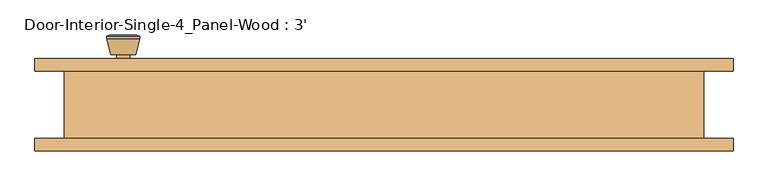
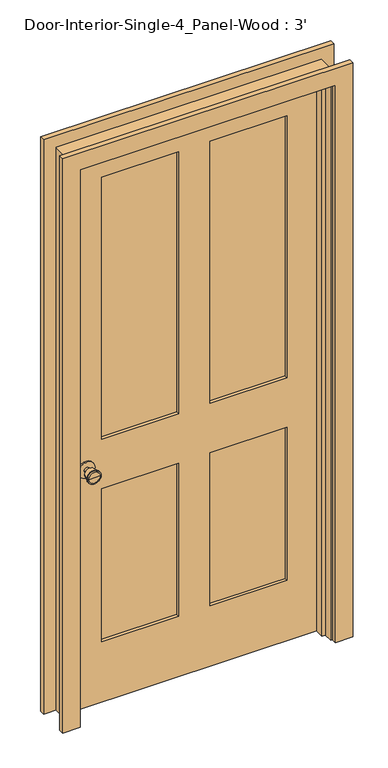
"""IFC4 building model written with IfcOpenShell, lengths in millimetres: door geometry, Door-Interior-Single-4_Panel-Wood : 3'."""

from ifc_helpers import new_model, si_unit, point, frame, frame_2d, origin, place, context, project, spatial, polyline, circle_curve, trimmed, segment, composite_curve, outline, extrude, faceted_brep, source, transform, mapped, element, save
from ifc_brep_helpers import plane_surface, cylinder_surface, revolved_surface, advanced_brep


def door_interior_single_4_panel_wood_3_aef61117(model_context):
    return source(origin(), model_context, "Body", "SolidModel", [
        advanced_brep(
        [(-393.7, 6.7, 914.4), (-383.7, 6.7, 914.4), (-403.7, 6.7, 914.4), (-373.2241324, -42.3, 914.4), (-393.7, -42.3, 914.4), (-414.1758676, -42.3, 914.4), (-368.7, -40.4721319, 914.4), (-418.7, -40.4721319, 914.4), (-368.7, -37.0084537, 914.4), (-418.7, -37.0084537, 914.4), (-375.063764, -12.3, 914.4), (-412.336236, -12.3, 914.4), (-383.7, -12.3, 914.4), (-403.7, -12.3, 914.4)],
        [
            (0, 1),
            (1, 2, circle_curve(frame((-393.7, 6.7, 914.4), z_axis=(0.0, 1.0, 0.0), x_axis=(-1.0, 0.0, 0.0)), 10.0)),
            (2, 0),
            (2, 1, circle_curve(frame((-393.7, 6.7, 914.4), z_axis=(0.0, 1.0, 0.0), x_axis=(-1.0, 0.0, 0.0)), 10.0)),
            (3, 4),
            (4, 5),
            (5, 3, circle_curve(frame((-393.7, -42.3, 914.4), z_axis=(0.0, -1.0, 0.0), x_axis=(-1.0, 0.0, 0.0)), 20.4758676)),
            (3, 5, circle_curve(frame((-393.7, -42.3, 914.4), z_axis=(0.0, -1.0, 0.0), x_axis=(-1.0, 0.0, 0.0)), 20.4758676)),
            (6, 3),
            (5, 7),
            (7, 6, circle_curve(frame((-393.7, -40.4721319, 914.4), z_axis=(0.0, -1.0, 0.0), x_axis=(-1.0, 0.0, 0.0)), 25.0)),
            (6, 7, circle_curve(frame((-393.7, -40.4721319, 914.4), z_axis=(0.0, -1.0, 0.0), x_axis=(-1.0, 0.0, 0.0)), 25.0)),
            (8, 6),
            (7, 9),
            (9, 8, circle_curve(frame((-393.7, -37.0084537, 914.4), z_axis=(0.0, -1.0, 0.0), x_axis=(-1.0, 0.0, 0.0)), 25.0)),
            (8, 9, circle_curve(frame((-393.7, -37.0084537, 914.4), z_axis=(0.0, -1.0, 0.0), x_axis=(-1.0, 0.0, 0.0)), 25.0)),
            (10, 8),
            (9, 11),
            (11, 10, circle_curve(frame((-393.7, -12.3, 914.4), z_axis=(0.0, -1.0, 0.0), x_axis=(-1.0, 0.0, 0.0)), 18.636236)),
            (10, 11, circle_curve(frame((-393.7, -12.3, 914.4), z_axis=(0.0, -1.0, 0.0), x_axis=(-1.0, 0.0, 0.0)), 18.636236)),
            (12, 10),
            (11, 13),
            (13, 12, circle_curve(frame((-393.7, -12.3, 914.4), z_axis=(0.0, -1.0, 0.0), x_axis=(-1.0, 0.0, 0.0)), 10.0)),
            (12, 13, circle_curve(frame((-393.7, -12.3, 914.4), z_axis=(0.0, -1.0, 0.0), x_axis=(-1.0, 0.0, 0.0)), 10.0)),
            (1, 12),
            (13, 2),
        ],
        [
            plane_surface(frame((-393.7, 6.7, 914.4), z_axis=(0.0, 1.0, 0.0), x_axis=(-1.0, 0.0, 0.0))),
            plane_surface(frame((-393.7, -42.3, 914.4), z_axis=(0.0, -1.0, 0.0), x_axis=(-1.0, 0.0, 0.0))),
            revolved_surface(polyline([(-414.1758676, -42.3, 914.4), (-418.7, -40.4721319, 914.4)]), (-393.7, 6.7, 914.4), (0.0, 1.0, 0.0)),
            cylinder_surface(frame((-393.7, 6.7, 914.4), z_axis=(0.0, 1.0, 0.0), x_axis=(-1.0, 0.0, 0.0)), 25.0),
            revolved_surface(polyline([(-418.7, -37.0084537, 914.4), (-412.336236, -12.3, 914.4)]), (-393.7, 6.7, 914.4), (0.0, 1.0, 0.0)),
            plane_surface(frame((-393.7, -12.3, 914.4), z_axis=(0.0, 1.0, 0.0), x_axis=(-1.0, 0.0, 0.0))),
            cylinder_surface(frame((-393.7, 6.7, 914.4), z_axis=(0.0, 1.0, 0.0), x_axis=(-1.0, 0.0, 0.0)), 10.0),
        ],
        [
            (0, [[1, 2, 3]]),
            (0, [[-3, 4, -1]]),
            (1, [[5, 6, 7]]),
            (1, [[-6, -5, 8]]),
            (2, [[9, -7, 10, 11]]),
            (2, [[-10, -8, -9, 12]]),
            (3, [[13, -11, 14, 15]]),
            (3, [[-14, -12, -13, 16]]),
            (4, [[17, -15, 18, 19]]),
            (4, [[-18, -16, -17, 20]]),
            (5, [[21, -19, 22, 23]]),
            (5, [[-22, -20, -21, 24]]),
            (6, [[25, -23, 26, -2]]),
            (6, [[-26, -24, -25, -4]]),
        ],
    ),
        extrude(outline(composite_curve([segment(trimmed(circle_curve(frame_2d((914.4, -393.7)), 30.0), [point((914.4, -423.7))], [point((914.4, -363.7))], False, "CARTESIAN"), True, "CONTINUOUS"), segment(trimmed(circle_curve(frame_2d((914.4, -393.7)), 30.0), [point((914.4, -363.7))], [point((914.4, -423.7))], False, "CARTESIAN"), True, "CONTINUOUS")], self_intersect=False)), frame((0.0, 6.7, 0.0), z_axis=(0.0, 1.0, 0.0), x_axis=(0.0, 0.0, 1.0)), (0.0, 0.0, 1.0), 6.0),
        advanced_brep(
        [(-393.7, 53.625, 914.4), (-403.7, 53.625, 914.4), (-383.7, 53.625, 914.4), (-373.2241324, 102.625, 914.4), (-414.1758676, 102.625, 914.4), (-393.7, 102.625, 914.4), (-368.7, 100.7971319, 914.4), (-418.7, 100.7971319, 914.4), (-368.7, 97.3334537, 914.4), (-418.7, 97.3334537, 914.4), (-375.063764, 72.625, 914.4), (-412.336236, 72.625, 914.4), (-383.7, 72.625, 914.4), (-403.7, 72.625, 914.4)],
        [
            (0, 1),
            (1, 2, circle_curve(frame((-393.7, 53.625, 914.4), z_axis=(0.0, -1.0, 0.0), x_axis=(-1.0, 0.0, 0.0)), 10.0)),
            (2, 0),
            (2, 1, circle_curve(frame((-393.7, 53.625, 914.4), z_axis=(0.0, -1.0, 0.0), x_axis=(-1.0, 0.0, 0.0)), 10.0)),
            (3, 4, circle_curve(frame((-393.7, 102.625, 914.4), z_axis=(0.0, 1.0, 0.0), x_axis=(-1.0, 0.0, 0.0)), 20.4758676)),
            (4, 5),
            (5, 3),
            (4, 3, circle_curve(frame((-393.7, 102.625, 914.4), z_axis=(0.0, 1.0, 0.0), x_axis=(-1.0, 0.0, 0.0)), 20.4758676)),
            (6, 7, circle_curve(frame((-393.7, 100.7971319, 914.4), z_axis=(0.0, 1.0, 0.0), x_axis=(-1.0, 0.0, 0.0)), 25.0)),
            (7, 4),
            (3, 6),
            (7, 6, circle_curve(frame((-393.7, 100.7971319, 914.4), z_axis=(0.0, 1.0, 0.0), x_axis=(-1.0, 0.0, 0.0)), 25.0)),
            (8, 9, circle_curve(frame((-393.7, 97.3334537, 914.4), z_axis=(0.0, 1.0, 0.0), x_axis=(-1.0, 0.0, 0.0)), 25.0)),
            (9, 7),
            (6, 8),
            (9, 8, circle_curve(frame((-393.7, 97.3334537, 914.4), z_axis=(0.0, 1.0, 0.0), x_axis=(-1.0, 0.0, 0.0)), 25.0)),
            (10, 11, circle_curve(frame((-393.7, 72.625, 914.4), z_axis=(0.0, 1.0, 0.0), x_axis=(-1.0, 0.0, 0.0)), 18.636236)),
            (11, 9),
            (8, 10),
            (11, 10, circle_curve(frame((-393.7, 72.625, 914.4), z_axis=(0.0, 1.0, 0.0), x_axis=(-1.0, 0.0, 0.0)), 18.636236)),
            (12, 13, circle_curve(frame((-393.7, 72.625, 914.4), z_axis=(0.0, 1.0, 0.0), x_axis=(-1.0, 0.0, 0.0)), 10.0)),
            (13, 11),
            (10, 12),
            (13, 12, circle_curve(frame((-393.7, 72.625, 914.4), z_axis=(0.0, 1.0, 0.0), x_axis=(-1.0, 0.0, 0.0)), 10.0)),
            (1, 13),
            (12, 2),
        ],
        [
            plane_surface(frame((-393.7, 53.625, 914.4), z_axis=(0.0, -1.0, 0.0), x_axis=(-1.0, 0.0, 0.0))),
            plane_surface(frame((-393.7, 102.625, 914.4), z_axis=(0.0, 1.0, 0.0), x_axis=(-1.0, 0.0, 0.0))),
            revolved_surface(polyline([(-414.1758676, 102.625, 914.4), (-418.7, 100.7971319, 914.4)]), (-393.7, 53.625, 914.4), (0.0, -1.0, 0.0)),
            cylinder_surface(frame((-393.7, 53.625, 914.4), z_axis=(0.0, -1.0, 0.0), x_axis=(-1.0, 0.0, 0.0)), 25.0),
            revolved_surface(polyline([(-418.7, 97.3334537, 914.4), (-412.336236, 72.625, 914.4)]), (-393.7, 53.625, 914.4), (0.0, -1.0, 0.0)),
            plane_surface(frame((-393.7, 72.625, 914.4), z_axis=(0.0, -1.0, 0.0), x_axis=(-1.0, 0.0, 0.0))),
            cylinder_surface(frame((-393.7, 53.625, 914.4), z_axis=(0.0, -1.0, 0.0), x_axis=(-1.0, 0.0, 0.0)), 10.0),
        ],
        [
            (0, [[1, 2, 3]]),
            (0, [[-3, 4, -1]]),
            (1, [[5, 6, 7]]),
            (1, [[8, -7, -6]]),
            (2, [[9, 10, -5, 11]]),
            (2, [[12, -11, -8, -10]]),
            (3, [[13, 14, -9, 15]]),
            (3, [[16, -15, -12, -14]]),
            (4, [[17, 18, -13, 19]]),
            (4, [[20, -19, -16, -18]]),
            (5, [[21, 22, -17, 23]]),
            (5, [[24, -23, -20, -22]]),
            (6, [[-2, 25, -21, 26]]),
            (6, [[-4, -26, -24, -25]]),
        ],
    ),
        extrude(outline(composite_curve([segment(trimmed(circle_curve(frame_2d((914.4, -393.7)), 30.0), [point((914.4, -423.7))], [point((914.4, -363.7))], False, "CARTESIAN"), True, "CONTINUOUS"), segment(trimmed(circle_curve(frame_2d((914.4, -393.7)), 30.0), [point((914.4, -363.7))], [point((914.4, -423.7))], False, "CARTESIAN"), True, "CONTINUOUS")], self_intersect=False)), frame((0.0, 47.625, 0.0), z_axis=(0.0, 1.0, 0.0), x_axis=(0.0, 0.0, 1.0)), (0.0, 0.0, 1.0), 6.0),
        extrude(outline(polyline([(336.55, 24.3416667), (57.15, 24.3416667), (57.15, 35.9833333), (336.55, 35.9833333), (336.55, 24.3416667)])), frame((0.0, 0.0, 1009.65), z_axis=(0.0, 0.0, 1.0), x_axis=(1.0, 0.0, 0.0)), (0.0, 0.0, 1.0), 1004.8875),
        extrude(outline(polyline([(-57.15, 24.3416667), (-336.55, 24.3416667), (-336.55, 35.9833333), (-57.15, 35.9833333), (-57.15, 24.3416667)])), frame((0.0, 0.0, 1009.65), z_axis=(0.0, 0.0, 1.0), x_axis=(1.0, 0.0, 0.0)), (0.0, 0.0, 1.0), 1004.8875),
        extrude(outline(polyline([(336.55, 24.3416667), (57.15, 24.3416667), (57.15, 35.9833333), (336.55, 35.9833333), (336.55, 24.3416667)])), frame((0.0, 0.0, 231.775), z_axis=(0.0, 0.0, 1.0), x_axis=(1.0, 0.0, 0.0)), (0.0, 0.0, 1.0), 587.375),
        extrude(outline(polyline([(-57.15, 24.3416667), (-336.55, 24.3416667), (-336.55, 35.9833333), (-57.15, 35.9833333), (-57.15, 24.3416667)])), frame((0.0, 0.0, 231.775), z_axis=(0.0, 0.0, 1.0), x_axis=(1.0, 0.0, 0.0)), (0.0, 0.0, 1.0), 587.375),
        extrude(outline(polyline([(2133.6, -457.2), (0.0, -457.2), (0.0, 457.2), (2133.6, 457.2), (2133.6, -457.2)]), holes=[polyline([(2014.5375, 57.15), (2014.5375, 336.55), (1009.65, 336.55), (1009.65, 57.15), (2014.5375, 57.15)]), polyline([(1009.65, -57.15), (1009.65, -336.55), (2014.5375, -336.55), (2014.5375, -57.15), (1009.65, -57.15)]), polyline([(819.15, 57.15), (819.15, 336.55), (231.775, 336.55), (231.775, 57.15), (819.15, 57.15)]), polyline([(231.775, -57.15), (231.775, -336.55), (819.15, -336.55), (819.15, -57.15), (231.775, -57.15)])]), frame((0.0, 12.7, 0.0), z_axis=(0.0, 1.0, 0.0), x_axis=(0.0, 0.0, 1.0)), (0.0, 0.0, 1.0), 34.925),
        faceted_brep([(482.6, 47.625, 0.0), (482.6, -53.975, 0.0), (457.2, -53.975, 0.0), (457.2, -22.225, 0.0), (444.5, -22.225, 0.0), (444.5, 12.7, 0.0), (457.2, 12.7, 0.0), (457.2, 47.625, 0.0), (482.6, 47.625, 2159.0), (482.6, -53.975, 2159.0), (-482.6, -53.975, 2159.0), (-482.6, -53.975, 0.0), (-457.2, -53.975, 0.0), (-457.2, -53.975, 2133.6), (457.2, -53.975, 2133.6), (457.2, -22.225, 2133.6), (-457.2, -22.225, 2133.6), (-457.2, -22.225, 0.0), (-444.5, -22.225, 0.0), (-444.5, -22.225, 2120.9), (444.5, -22.225, 2120.9), (444.5, 12.7, 2120.9), (-444.5, 12.7, 2120.9), (-444.5, 12.7, 0.0), (-457.2, 12.7, 0.0), (-457.2, 12.7, 2133.6), (457.2, 12.7, 2133.6), (457.2, 47.625, 2133.6), (-457.2, 47.625, 2133.6), (-457.2, 47.625, 0.0), (-482.6, 47.625, 0.0), (-482.6, 47.625, 2159.0)], [[[0, 1, 2, 3, 4, 5, 6, 7]], [[1, 0, 8, 9]], [[2, 1, 9, 10, 11, 12, 13, 14]], [[3, 2, 14, 15]], [[4, 3, 15, 16, 17, 18, 19, 20]], [[5, 4, 20, 21]], [[6, 5, 21, 22, 23, 24, 25, 26]], [[7, 6, 26, 27]], [[0, 7, 27, 28, 29, 30, 31, 8]], [[9, 8, 31, 10]], [[15, 14, 13, 16]], [[21, 20, 19, 22]], [[27, 26, 25, 28]], [[30, 29, 24, 23, 18, 17, 12, 11]], [[10, 31, 30, 11]], [[16, 13, 12, 17]], [[22, 19, 18, 23]], [[28, 25, 24, 29]]]),
        extrude(outline(polyline([(0.0, 463.55), (0.0, 527.05), (2203.45, 527.05), (2203.45, -527.05), (0.0, -527.05), (0.0, -463.55), (2139.95, -463.55), (2139.95, 463.55), (0.0, 463.55)])), frame((0.0, -73.025, 0.0), z_axis=(0.0, 1.0, 0.0), x_axis=(0.0, 0.0, 1.0)), (0.0, 0.0, 1.0), 19.05),
        extrude(outline(polyline([(0.0, 463.55), (0.0, 527.05), (2203.45, 527.05), (2203.45, -527.05), (0.0, -527.05), (0.0, -463.55), (2139.95, -463.55), (2139.95, 463.55), (0.0, 463.55)])), frame((0.0, 47.625, 0.0), z_axis=(0.0, 1.0, 0.0), x_axis=(0.0, 0.0, 1.0)), (0.0, 0.0, 1.0), 19.05),
    ])


if __name__ == "__main__":
    model = new_model("IFC4")
    model_context = context("Model", 3, world=origin())
    ifc_project = project(units=[si_unit("LENGTHUNIT", "METRE", prefix="MILLI")], contexts=[model_context])
    site = spatial("IfcSite", under=ifc_project)
    building = spatial("IfcBuilding", under=site)
    placement = place(None, origin())
    door_interior_single_4_panel_wood_3_shape = door_interior_single_4_panel_wood_3_aef61117(model_context)
    element("IfcDoor", 1, ObjectType="Door-Interior-Single-4_Panel-Wood : 3'", at=placement, inside=building, context=model_context, shape_type="MappedRepresentation", body=[
        mapped(door_interior_single_4_panel_wood_3_shape, transform((0.0, 0.0, 0.0), x_axis=(1.0, 0.0, 0.0), y_axis=(0.0, 1.0, 0.0), z_axis=(0.0, 0.0, 1.0))),
    ])
    save(model, "model.ifc")

# Revit data of these elements
# Type "Door-Interior-Single-4_Panel-Wood : 3'"
#   Type Mark = "11"
#   Assembly Code = "C1020300"
#   Analytic Construction = "Wooden"
#   Top Rail = 0' - 4 11/16"
#   Thickness = 0' - 1 3/8"
#   Thermal Resistance (R) = 2.5876 (h·ft²·°F)/BTU
#   Swing Angle [instance default] = 90.00°
#   Stiles = 0' - 4 3/4"
#   Rough Width = 3' - 2"
#   Rough Height = 7' - 1"
#   Mullion = 0' - 4 1/2"
#   Lock Rail = 0' - 7 1/2"
#   Height = 7' - 0"
#   Width = 3' - 0"
#   Heat Transfer Coefficient (U) = 0.3865 BTU/(h·ft²·°F)
#   Bottom Rail = 0' - 9 1/8"
#   Trim Material = Cherry
#   Panel Material = Cherry
#   Frame Material = Cherry
#   Door Handle Material = Aluminum
#   Visual Light Transmittance = 0
#   Solar Heat Gain Coefficient = 0
#   Wall Closure = (empty or 0)
#   Function = (empty or 0)
# Element 1 (IfcDoor, "Door-Interior-Single-4_Panel-Wood : 3'")
#   Materials on its faces: "Cherry", "Aluminum"
# Materials
#   "Cherry": class "Wood", colour RGB 226 177 128, transparency 0, Description = "Prunus Serotina", Cost = 0
#   "Aluminum": class "Metal", colour RGB 247 247 247, transparency 0, Description = "Aluminum 6061", Cost = 0
